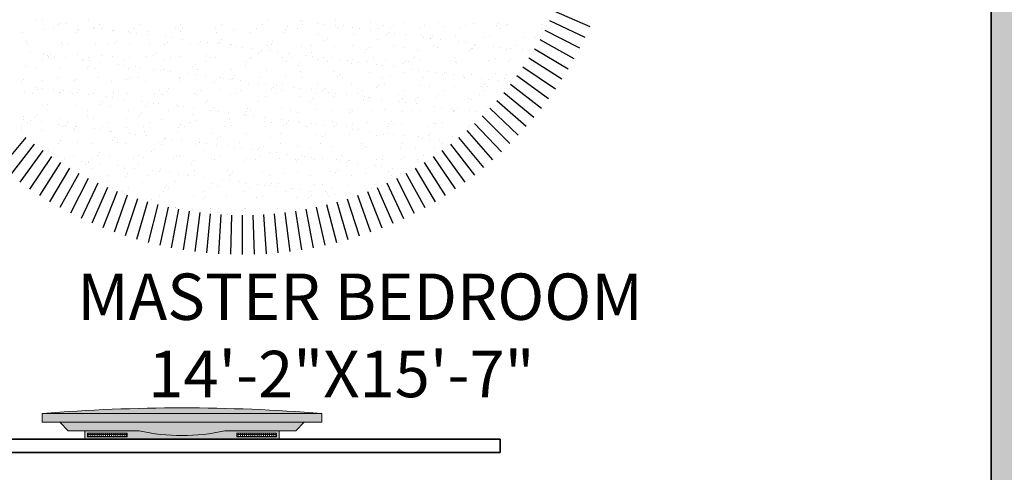
# Model space of a CAD drawing. Units: inches. Extents: x 1566 to 2546, y 1087 to 2705.
# Tile 21 of 27: x 2130 to 2278, y 1625 to 1694. Entities that reach past the tile are written whole.
import ezdxf

# ---------------------------------------------------------------- set-up
doc = ezdxf.new("R2010")
doc.units = ezdxf.units.IN
for name, color, linetype, lineweight in [('A-AREA-IDEN', 7, 'Continuous', 18), ('A-FURN', 8, 'Continuous', 18), ('A-WALL', 7, 'Continuous', 35), ('A-WALL-PATT', 8, 'Continuous', 13), ('moveis', 254, 'Continuous', 5), ('parede', 7, 'Continuous', 30)]:
    doc.layers.add(name, color=color, linetype=linetype, lineweight=lineweight)
doc.layers.add('A-HT', color=15, linetype='Continuous')
doc.styles.get("Standard").update_dxf_attribs({"font": 'arial.ttf'})

# ---------------------------------------------------------------- blocks, each defined once
blk = doc.blocks.new('*X21')
at = {"color": 0}
for p, q in [((1.8017, 2.833), (1.8017, 2.833)), ((1.8783, 2.8364), (1.8783, 2.8364)), ((1.9044, 2.8399), (1.9044, 2.8399)), ((1.945, 2.8452), (1.945, 2.8452)), ((2.0018, 2.8313), (2.0018, 2.8313)), ((1.7428, 2.8186), (1.7428, 2.8186)), ((1.7438, 2.8187), (1.7438, 2.8187)), ((1.7537, 2.8227), (1.7537, 2.8227)), ((1.7698, 2.8221), (1.7698, 2.8221)), ((1.8104, 2.8275), (1.8104, 2.8275)), ((1.8778, 2.8235), (1.8778, 2.8235)), ((1.9094, 2.823), (1.9094, 2.823)), ((2.0087, 2.8252), (2.0087, 2.8252)), ((2.011, 2.8229), (2.011, 2.8229)), ((2.0652, 2.8233), (2.0652, 2.8233)), ((2.1366, 2.8246), (2.1366, 2.8246)), ((2.2048, 2.8269), (2.2048, 2.8269)), ((2.2209, 2.8236), (2.2209, 2.8236)), ((1.5414, 2.759), (1.5414, 2.759)), ((1.5474, 2.7675), (1.5474, 2.7675)), ((1.6514, 2.7891), (1.6514, 2.7891)), ((1.6825, 2.7724), (1.6825, 2.7724)), ((1.6971, 2.7593), (1.6971, 2.7593)), ((1.8133, 2.774), (1.8133, 2.774)), ((1.8515, 2.7874), (1.8515, 2.7874)), ((1.8528, 2.7596), (1.8528, 2.7596)), ((1.8607, 2.779), (1.8607, 2.779)), ((1.9412, 2.7734), (1.9412, 2.7734)), ((2.0085, 2.7599), (2.0085, 2.7599)), ((2.0545, 2.783), (2.0545, 2.783)), ((2.0763, 2.7783), (2.0763, 2.7783)), ((2.1643, 2.7602), (2.1643, 2.7602)), ((2.2072, 2.78), (2.2072, 2.78)), ((2.2546, 2.7813), (2.2546, 2.7813)), ((2.2603, 2.7573), (2.2603, 2.7573)), ((2.2638, 2.7728), (2.2638, 2.7728)), ((2.32, 2.7605), (2.32, 2.7605)), ((2.3282, 2.7662), (2.3282, 2.7662)), ((2.3351, 2.7793), (2.3351, 2.7793)), ((2.3542, 2.7696), (2.3542, 2.7696)), ((2.3949, 2.775), (2.3949, 2.775)), ((1.4871, 2.7212), (1.4871, 2.7212)), ((1.5011, 2.7453), (1.5011, 2.7453)), ((1.5625, 2.7456), (1.5625, 2.7456)), ((1.618, 2.7229), (1.618, 2.7229)), ((1.7012, 2.7435), (1.7012, 2.7435)), ((1.7104, 2.7351), (1.7104, 2.7351)), ((1.7182, 2.7459), (1.7182, 2.7459)), ((1.7459, 2.7223), (1.7459, 2.7223)), ((1.8739, 2.7462), (1.8739, 2.7462)), ((1.881, 2.7272), (1.881, 2.7272)), ((1.9042, 2.7391), (1.9042, 2.7391)), ((1.9505, 2.7165), (1.9505, 2.7165)), ((1.9911, 2.7218), (1.9911, 2.7218)), ((2.0118, 2.7288), (2.0118, 2.7288)), ((2.0296, 2.7465), (2.0296, 2.7465)), ((2.059, 2.7308), (2.059, 2.7308)), ((2.0851, 2.7342), (2.0851, 2.7342)), ((2.1043, 2.7374), (2.1043, 2.7374)), ((2.1135, 2.729), (2.1135, 2.729)), ((2.1257, 2.7395), (2.1257, 2.7395)), ((2.1397, 2.7282), (2.1397, 2.7282)), ((2.1853, 2.7467), (2.1853, 2.7467)), ((2.1936, 2.7485), (2.1936, 2.7485)), ((2.2196, 2.7519), (2.2196, 2.7519)), ((2.2748, 2.7331), (2.2748, 2.7331)), ((2.3073, 2.733), (2.3073, 2.733)), ((2.341, 2.747), (2.341, 2.747)), ((2.4057, 2.7348), (2.4057, 2.7348)), ((2.4967, 2.7473), (2.4967, 2.7473)), ((2.5074, 2.7313), (2.5074, 2.7313)), ((2.5166, 2.7228), (2.5166, 2.7228)), ((2.5336, 2.7341), (2.5336, 2.7341)), ((1.4827, 2.697), (1.4827, 2.697)), ((1.5509, 2.6997), (1.5509, 2.6997)), ((1.5601, 2.6912), (1.5601, 2.6912)), ((1.6384, 2.6973), (1.6384, 2.6973)), ((1.6553, 2.6776), (1.6553, 2.6776)), ((1.6813, 2.681), (1.6813, 2.681)), ((1.7219, 2.6864), (1.7219, 2.6864)), ((1.7539, 2.6952), (1.7539, 2.6952)), ((1.7899, 2.6953), (1.7899, 2.6953)), ((1.7941, 2.6975), (1.7941, 2.6975)), ((1.8159, 2.6988), (1.8159, 2.6988)), ((1.8165, 2.6777), (1.8165, 2.6777)), ((1.8565, 2.7041), (1.8565, 2.7041)), ((1.9244, 2.7131), (1.9244, 2.7131)), ((1.9498, 2.6978), (1.9498, 2.6978)), ((1.954, 2.6935), (1.954, 2.6935)), ((1.9632, 2.6851), (1.9632, 2.6851)), ((2.0794, 2.682), (2.0794, 2.682)), ((2.1055, 2.6981), (2.1055, 2.6981)), ((2.157, 2.6891), (2.157, 2.6891)), ((2.2103, 2.6836), (2.2103, 2.6836)), ((2.2612, 2.6984), (2.2612, 2.6984)), ((2.3382, 2.683), (2.3382, 2.683)), ((2.3571, 2.6874), (2.3571, 2.6874)), ((2.3663, 2.6789), (2.3663, 2.6789)), ((2.4169, 2.6987), (2.4169, 2.6987)), ((2.4733, 2.6879), (2.4733, 2.6879)), ((2.5601, 2.683), (2.5601, 2.683)), ((2.5727, 2.6989), (2.5727, 2.6989)), ((2.6042, 2.6895), (2.6042, 2.6895)), ((2.6435, 2.6783), (2.6435, 2.6783)), ((1.3861, 2.6422), (1.3861, 2.6422)), ((1.4006, 2.6558), (1.4006, 2.6558)), ((1.4098, 2.6473), (1.4098, 2.6473)), ((1.4121, 2.6456), (1.4121, 2.6456)), ((1.4227, 2.6718), (1.4227, 2.6718)), ((1.4528, 2.651), (1.4528, 2.651)), ((1.5207, 2.6599), (1.5207, 2.6599)), ((1.5467, 2.6633), (1.5467, 2.6633)), ((1.5506, 2.6712), (1.5506, 2.6712)), ((1.5873, 2.6687), (1.5873, 2.6687)), ((1.6036, 2.6513), (1.6036, 2.6513)), ((1.6856, 2.676), (1.6856, 2.676)), ((1.8037, 2.6496), (1.8037, 2.6496)), ((1.8129, 2.6412), (1.8129, 2.6412)), ((1.9444, 2.6771), (1.9444, 2.6771)), ((2.0067, 2.6452), (2.0067, 2.6452)), ((2.2068, 2.6435), (2.2068, 2.6435)), ((2.3743, 2.6428), (2.3743, 2.6428)), ((2.4003, 2.6462), (2.4003, 2.6462)), ((2.441, 2.6516), (2.441, 2.6516)), ((2.5089, 2.6605), (2.5089, 2.6605)), ((2.5349, 2.664), (2.5349, 2.664)), ((2.5756, 2.6693), (2.5756, 2.6693)), ((2.6718, 2.6427), (2.6718, 2.6427)), ((1.2503, 2.6119), (1.2503, 2.6119)), ((1.2595, 2.6034), (1.2595, 2.6034)), ((1.2775, 2.6279), (1.2775, 2.6279)), ((1.2915, 2.6198), (1.2915, 2.6198)), ((1.3182, 2.6332), (1.3182, 2.6332)), ((1.3552, 2.62), (1.3552, 2.62)), ((1.4261, 2.6336), (1.4261, 2.6336)), ((1.4472, 2.6201), (1.4472, 2.6201)), ((1.4533, 2.6075), (1.4533, 2.6075)), ((1.4903, 2.6249), (1.4903, 2.6249)), ((1.5818, 2.6338), (1.5818, 2.6338)), ((1.6029, 2.6204), (1.6029, 2.6204)), ((1.6212, 2.6266), (1.6212, 2.6266)), ((1.6534, 2.6057), (1.6534, 2.6057)), ((1.7375, 2.6341), (1.7375, 2.6341)), ((1.7491, 2.626), (1.7491, 2.626)), ((1.7586, 2.6207), (1.7586, 2.6207)), ((1.8841, 2.6308), (1.8841, 2.6308)), ((1.8932, 2.6344), (1.8932, 2.6344)), ((1.9143, 2.621), (1.9143, 2.621)), ((2.015, 2.6325), (2.015, 2.6325)), ((2.0489, 2.6347), (2.0489, 2.6347)), ((2.07, 2.6213), (2.07, 2.6213)), ((2.1051, 2.6074), (2.1051, 2.6074)), ((2.1312, 2.6108), (2.1312, 2.6108)), ((2.1429, 2.6319), (2.1429, 2.6319)), ((2.1718, 2.6162), (2.1718, 2.6162)), ((2.2046, 2.635), (2.2046, 2.635)), ((2.216, 2.635), (2.216, 2.635)), ((2.2257, 2.6215), (2.2257, 2.6215)), ((2.2397, 2.6251), (2.2397, 2.6251)), ((2.2657, 2.6285), (2.2657, 2.6285)), ((2.2779, 2.6367), (2.2779, 2.6367)), ((2.3064, 2.6339), (2.3064, 2.6339)), ((2.3603, 2.6352), (2.3603, 2.6352)), ((2.3814, 2.6218), (2.3814, 2.6218)), ((2.4088, 2.6384), (2.4088, 2.6384)), ((2.4098, 2.6391), (2.4098, 2.6391)), ((2.516, 2.6355), (2.516, 2.6355)), ((2.5367, 2.6378), (2.5367, 2.6378)), ((2.5371, 2.6221), (2.5371, 2.6221)), ((2.6099, 2.6374), (2.6099, 2.6374)), ((2.6191, 2.6289), (2.6191, 2.6289)), ((2.6718, 2.6358), (2.6718, 2.6358)), ((2.6928, 2.6224), (2.6928, 2.6224)), ((1.2117, 2.5712), (1.2117, 2.5712)), ((1.2949, 2.5738), (1.2949, 2.5738)), ((1.3674, 2.5715), (1.3674, 2.5715)), ((1.4258, 2.5754), (1.4258, 2.5754)), ((1.5231, 2.5718), (1.5231, 2.5718)), ((1.5537, 2.5748), (1.5537, 2.5748)), ((1.6626, 2.5973), (1.6626, 2.5973)), ((1.6788, 2.572), (1.6788, 2.572)), ((1.6888, 2.5797), (1.6888, 2.5797)), ((1.8196, 2.5814), (1.8196, 2.5814)), ((1.8345, 2.5723), (1.8345, 2.5723)), ((1.836, 2.5719), (1.836, 2.5719)), ((1.8564, 2.6013), (1.8564, 2.6013)), ((1.862, 2.5754), (1.862, 2.5754)), ((1.9026, 2.5807), (1.9026, 2.5807)), ((1.9475, 2.5807), (1.9475, 2.5807)), ((1.9705, 2.5897), (1.9705, 2.5897)), ((1.9902, 2.5726), (1.9902, 2.5726)), ((1.9966, 2.5931), (1.9966, 2.5931)), ((2.0372, 2.5984), (2.0372, 2.5984)), ((2.0565, 2.5996), (2.0565, 2.5996)), ((2.0657, 2.5912), (2.0657, 2.5912)), ((2.0826, 2.5856), (2.0826, 2.5856)), ((2.1459, 2.5729), (2.1459, 2.5729)), ((2.2135, 2.5873), (2.2135, 2.5873)), ((2.2595, 2.5952), (2.2595, 2.5952)), ((2.3016, 2.5732), (2.3016, 2.5732)), ((2.3414, 2.5867), (2.3414, 2.5867)), ((2.4573, 2.5735), (2.4573, 2.5735)), ((2.4595, 2.5935), (2.4595, 2.5935)), ((2.4688, 2.585), (2.4688, 2.585)), ((2.4764, 2.5915), (2.4764, 2.5915)), ((2.6073, 2.5932), (2.6073, 2.5932)), ((2.613, 2.5737), (2.613, 2.5737)), ((2.6626, 2.589), (2.6626, 2.589)), ((2.7352, 2.5926), (2.7352, 2.5926)), ((2.7687, 2.574), (2.7687, 2.574)), ((1.303, 2.5636), (1.303, 2.5636)), ((1.4934, 2.5286), (1.4934, 2.5286)), ((1.4989, 2.5276), (1.4989, 2.5276)), ((1.5031, 2.5619), (1.5031, 2.5619)), ((1.5123, 2.5534), (1.5123, 2.5534)), ((1.5668, 2.5365), (1.5668, 2.5365)), ((1.5928, 2.5399), (1.5928, 2.5399)), ((1.6243, 2.5302), (1.6243, 2.5302)), ((1.6334, 2.5453), (1.6334, 2.5453)), ((1.7014, 2.5542), (1.7014, 2.5542)), ((1.7061, 2.5574), (1.7061, 2.5574)), ((1.7274, 2.5577), (1.7274, 2.5577)), ((1.7522, 2.5296), (1.7522, 2.5296)), ((1.768, 2.563), (1.768, 2.563)), ((1.8873, 2.5345), (1.8873, 2.5345)), ((1.9061, 2.5557), (1.9061, 2.5557)), ((1.9154, 2.5473), (1.9154, 2.5473)), ((2.0181, 2.5361), (2.0181, 2.5361)), ((2.1092, 2.5513), (2.1092, 2.5513)), ((2.146, 2.5355), (2.146, 2.5355)), ((2.2811, 2.5404), (2.2811, 2.5404)), ((2.3092, 2.5496), (2.3092, 2.5496)), ((2.3185, 2.5411), (2.3185, 2.5411)), ((2.412, 2.5421), (2.412, 2.5421)), ((2.4871, 2.5282), (2.4871, 2.5282)), ((2.5123, 2.5452), (2.5123, 2.5452)), ((2.5399, 2.5415), (2.5399, 2.5415)), ((2.555, 2.5371), (2.555, 2.5371)), ((2.581, 2.5406), (2.581, 2.5406)), ((2.6217, 2.5459), (2.6217, 2.5459)), ((2.6749, 2.5463), (2.6749, 2.5463)), ((2.6896, 2.5549), (2.6896, 2.5549)), ((2.7123, 2.5434), (2.7123, 2.5434)), ((2.7156, 2.5583), (2.7156, 2.5583)), ((2.7216, 2.535), (2.7216, 2.535)), ((2.7563, 2.5636), (2.7563, 2.5636)), ((2.8058, 2.548), (2.8058, 2.548)), ((1.1527, 2.5197), (1.1527, 2.5197)), ((1.1551, 2.5078), (1.1551, 2.5078)), ((1.1761, 2.4943), (1.1761, 2.4943)), ((1.2297, 2.4921), (1.2297, 2.4921)), ((1.2305, 2.5243), (1.2305, 2.5243)), ((1.2976, 2.5011), (1.2976, 2.5011)), ((1.3108, 2.5081), (1.3108, 2.5081)), ((1.3236, 2.5045), (1.3236, 2.5045)), ((1.3319, 2.4946), (1.3319, 2.4946)), ((1.3527, 2.518), (1.3527, 2.518)), ((1.3584, 2.5237), (1.3584, 2.5237)), ((1.362, 2.5095), (1.362, 2.5095)), ((1.3643, 2.5098), (1.3643, 2.5098)), ((1.4322, 2.5188), (1.4322, 2.5188)), ((1.4582, 2.5222), (1.4582, 2.5222)), ((1.4665, 2.5083), (1.4665, 2.5083)), ((1.4876, 2.4949), (1.4876, 2.4949)), ((1.5558, 2.5136), (1.5558, 2.5136)), ((1.6222, 2.5086), (1.6222, 2.5086)), ((1.6433, 2.4952), (1.6433, 2.4952)), ((1.7558, 2.5118), (1.7558, 2.5118)), ((1.7651, 2.5034), (1.7651, 2.5034)), ((1.7779, 2.5089), (1.7779, 2.5089)), ((1.799, 2.4955), (1.799, 2.4955)), ((1.9336, 2.5092), (1.9336, 2.5092)), ((1.9547, 2.4958), (1.9547, 2.4958)), ((1.9589, 2.5074), (1.9589, 2.5074)), ((2.0857, 2.4893), (2.0857, 2.4893)), ((2.0893, 2.5095), (2.0893, 2.5095)), ((2.1104, 2.496), (2.1104, 2.496)), ((2.1589, 2.5057), (2.1589, 2.5057)), ((2.1682, 2.4973), (2.1682, 2.4973)), ((2.2166, 2.4909), (2.2166, 2.4909)), ((2.2179, 2.4928), (2.2179, 2.4928)), ((2.245, 2.5098), (2.245, 2.5098)), ((2.2661, 2.4963), (2.2661, 2.4963)), ((2.2858, 2.5017), (2.2858, 2.5017)), ((2.3118, 2.5051), (2.3118, 2.5051)), ((2.3445, 2.4903), (2.3445, 2.4903)), ((2.3525, 2.5105), (2.3525, 2.5105)), ((2.362, 2.5013), (2.362, 2.5013)), ((2.4007, 2.51), (2.4007, 2.51)), ((2.4204, 2.5194), (2.4204, 2.5194)), ((2.4218, 2.4966), (2.4218, 2.4966)), ((2.4464, 2.5229), (2.4464, 2.5229)), ((2.4796, 2.4952), (2.4796, 2.4952)), ((2.5564, 2.5103), (2.5564, 2.5103)), ((2.562, 2.4996), (2.562, 2.4996)), ((2.5712, 2.4911), (2.5712, 2.4911)), ((2.5775, 2.4969), (2.5775, 2.4969)), ((2.6104, 2.4969), (2.6104, 2.4969)), ((2.7121, 2.5106), (2.7121, 2.5106)), ((2.7332, 2.4972), (2.7332, 2.4972)), ((2.7384, 2.4962), (2.7384, 2.4962)), ((2.7651, 2.4951), (2.7651, 2.4951)), ((2.8678, 2.5109), (2.8678, 2.5109)), ((2.8734, 2.5011), (2.8734, 2.5011)), ((2.8889, 2.4975), (2.8889, 2.4975)), ((1.163, 2.4833), (1.163, 2.4833)), ((1.163, 2.4726), (1.163, 2.4726)), ((1.189, 2.4868), (1.189, 2.4868)), ((1.2024, 2.4741), (1.2024, 2.4741)), ((1.2117, 2.4657), (1.2117, 2.4657)), ((1.2981, 2.4774), (1.2981, 2.4774)), ((1.4055, 2.4697), (1.4055, 2.4697)), ((1.429, 2.4791), (1.429, 2.4791)), ((1.5569, 2.4785), (1.5569, 2.4785)), ((1.6055, 2.468), (1.6055, 2.468)), ((1.6148, 2.4595), (1.6148, 2.4595)), ((1.6919, 2.4833), (1.6919, 2.4833)), ((1.8086, 2.4635), (1.8086, 2.4635)), ((1.8228, 2.485), (1.8228, 2.485)), ((1.9081, 2.452), (1.9081, 2.452)), ((1.9487, 2.4573), (1.9487, 2.4573)), ((1.9507, 2.4844), (1.9507, 2.4844)), ((2.0086, 2.4618), (2.0086, 2.4618)), ((2.0166, 2.4663), (2.0166, 2.4663)), ((2.0178, 2.4534), (2.0178, 2.4534)), ((2.0427, 2.4697), (2.0427, 2.4697)), ((2.0833, 2.4751), (2.0833, 2.4751)), ((2.1512, 2.484), (2.1512, 2.484)), ((2.1773, 2.4874), (2.1773, 2.4874)), ((2.2117, 2.4574), (2.2117, 2.4574)), ((2.4117, 2.4557), (2.4117, 2.4557)), ((2.8089, 2.4516), (2.8089, 2.4516)), ((2.8963, 2.4526), (2.8963, 2.4526)), ((1.2336, 2.428), (1.2336, 2.428)), ((1.2521, 2.446), (1.2521, 2.446)), ((1.2552, 2.4258), (1.2552, 2.4258)), ((1.3615, 2.4273), (1.3615, 2.4273)), ((1.4078, 2.4463), (1.4078, 2.4463)), ((1.4552, 2.4241), (1.4552, 2.4241)), ((1.4644, 2.4156), (1.4644, 2.4156)), ((1.4966, 2.4322), (1.4966, 2.4322)), ((1.5635, 2.4466), (1.5635, 2.4466)), ((1.6275, 2.4339), (1.6275, 2.4339)), ((1.6389, 2.4165), (1.6389, 2.4165)), ((1.6582, 2.4197), (1.6582, 2.4197)), ((1.6795, 2.4219), (1.6795, 2.4219)), ((1.7192, 2.4468), (1.7192, 2.4468)), ((1.7475, 2.4308), (1.7475, 2.4308)), ((1.7554, 2.4333), (1.7554, 2.4333)), ((1.7735, 2.4343), (1.7735, 2.4343)), ((1.8141, 2.4396), (1.8141, 2.4396)), ((1.8583, 2.4179), (1.8583, 2.4179)), ((1.8749, 2.4471), (1.8749, 2.4471)), ((1.8821, 2.4486), (1.8821, 2.4486)), ((1.8904, 2.4381), (1.8904, 2.4381)), ((2.0213, 2.4398), (2.0213, 2.4398)), ((2.0306, 2.4474), (2.0306, 2.4474)), ((2.1492, 2.4392), (2.1492, 2.4392)), ((2.1863, 2.4477), (2.1863, 2.4477)), ((2.2842, 2.4441), (2.2842, 2.4441)), ((2.342, 2.448), (2.342, 2.448)), ((2.4151, 2.4457), (2.4151, 2.4457)), ((2.4209, 2.4472), (2.4209, 2.4472)), ((2.4977, 2.4483), (2.4977, 2.4483)), ((2.543, 2.4451), (2.543, 2.4451)), ((2.6011, 2.4138), (2.6011, 2.4138)), ((2.6147, 2.4513), (2.6147, 2.4513)), ((2.6271, 2.4172), (2.6271, 2.4172)), ((2.6534, 2.4485), (2.6534, 2.4485)), ((2.6678, 2.4225), (2.6678, 2.4225)), ((2.6781, 2.45), (2.6781, 2.45)), ((2.7357, 2.4315), (2.7357, 2.4315)), ((2.7617, 2.4349), (2.7617, 2.4349)), ((2.8024, 2.4403), (2.8024, 2.4403)), ((2.8091, 2.4488), (2.8091, 2.4488)), ((2.8148, 2.4495), (2.8148, 2.4495)), ((2.824, 2.4411), (2.824, 2.4411)), ((2.8703, 2.4492), (2.8703, 2.4492)), ((2.9368, 2.451), (2.9368, 2.451)), ((1.1662, 2.3762), (1.1662, 2.3762)), ((1.1954, 2.3826), (1.1954, 2.3826)), ((1.3012, 2.3811), (1.3012, 2.3811)), ((1.3049, 2.3802), (1.3049, 2.3802)), ((1.3437, 2.3777), (1.3437, 2.3777)), ((1.3512, 2.3829), (1.3512, 2.3829)), ((1.3697, 2.3811), (1.3697, 2.3811)), ((1.4104, 2.3865), (1.4104, 2.3865)), ((1.4321, 2.3828), (1.4321, 2.3828)), ((1.4783, 2.3954), (1.4783, 2.3954)), ((1.5043, 2.3988), (1.5043, 2.3988)), ((1.5069, 2.3831), (1.5069, 2.3831)), ((1.545, 2.4042), (1.545, 2.4042)), ((1.56, 2.3821), (1.56, 2.3821)), ((1.6129, 2.4131), (1.6129, 2.4131)), ((1.6626, 2.3834), (1.6626, 2.3834)), ((1.6951, 2.387), (1.6951, 2.387)), ((1.8183, 2.3837), (1.8183, 2.3837)), ((1.8259, 2.3887), (1.8259, 2.3887)), ((1.8675, 2.4095), (1.8675, 2.4095)), ((1.9538, 2.3881), (1.9538, 2.3881)), ((1.974, 2.384), (1.974, 2.384)), ((2.0613, 2.4135), (2.0613, 2.4135)), ((2.0889, 2.3929), (2.0889, 2.3929)), ((2.1297, 2.3843), (2.1297, 2.3843)), ((2.2198, 2.3946), (2.2198, 2.3946)), ((2.2614, 2.4118), (2.2614, 2.4118)), ((2.2706, 2.4033), (2.2706, 2.4033)), ((2.2854, 2.3846), (2.2854, 2.3846)), ((2.3319, 2.3783), (2.3319, 2.3783)), ((2.3477, 2.394), (2.3477, 2.394)), ((2.3579, 2.3817), (2.3579, 2.3817)), ((2.3986, 2.3871), (2.3986, 2.3871)), ((2.4411, 2.3848), (2.4411, 2.3848)), ((2.4644, 2.4074), (2.4644, 2.4074)), ((2.4665, 2.396), (2.4665, 2.396)), ((2.4827, 2.3988), (2.4827, 2.3988)), ((2.4925, 2.3995), (2.4925, 2.3995)), ((2.5332, 2.4048), (2.5332, 2.4048)), ((2.5968, 2.3851), (2.5968, 2.3851)), ((2.6136, 2.4005), (2.6136, 2.4005)), ((2.6645, 2.4057), (2.6645, 2.4057)), ((2.6737, 2.3972), (2.6737, 2.3972)), ((2.7415, 2.3999), (2.7415, 2.3999)), ((2.7525, 2.3854), (2.7525, 2.3854)), ((2.8675, 2.4012), (2.8675, 2.4012)), ((2.8765, 2.4048), (2.8765, 2.4048)), ((2.9082, 2.3857), (2.9082, 2.3857)), ((1.2091, 2.36), (1.2091, 2.36)), ((1.2165, 2.3691), (1.2165, 2.3691)), ((1.2351, 2.3634), (1.2351, 2.3634)), ((1.2758, 2.3687), (1.2758, 2.3687)), ((1.3141, 2.3717), (1.3141, 2.3717)), ((1.3722, 2.3694), (1.3722, 2.3694)), ((1.5079, 2.3758), (1.5079, 2.3758)), ((1.5279, 2.3697), (1.5279, 2.3697)), ((1.6837, 2.37), (1.6837, 2.37)), ((1.708, 2.374), (1.708, 2.374)), ((1.7172, 2.3656), (1.7172, 2.3656)), ((1.8394, 2.3703), (1.8394, 2.3703)), ((1.8936, 2.3418), (1.8936, 2.3418)), ((1.911, 2.3696), (1.911, 2.3696)), ((1.9951, 2.3706), (1.9951, 2.3706)), ((2.0244, 2.3435), (2.0244, 2.3435)), ((2.0627, 2.3429), (2.0627, 2.3429)), ((2.0888, 2.3463), (2.0888, 2.3463)), ((2.1111, 2.3679), (2.1111, 2.3679)), ((2.1203, 2.3595), (2.1203, 2.3595)), ((2.1294, 2.3517), (2.1294, 2.3517)), ((2.1508, 2.3708), (2.1508, 2.3708)), ((2.1523, 2.3429), (2.1523, 2.3429)), ((2.1973, 2.3606), (2.1973, 2.3606)), ((2.2234, 2.364), (2.2234, 2.364)), ((2.264, 2.3694), (2.264, 2.3694)), ((2.2874, 2.3477), (2.2874, 2.3477)), ((2.3065, 2.3711), (2.3065, 2.3711)), ((2.3141, 2.3635), (2.3141, 2.3635)), ((2.4183, 2.3494), (2.4183, 2.3494)), ((2.4622, 2.3714), (2.4622, 2.3714)), ((2.5142, 2.3618), (2.5142, 2.3618)), ((2.5234, 2.3533), (2.5234, 2.3533)), ((2.5462, 2.3488), (2.5462, 2.3488)), ((2.6179, 2.3717), (2.6179, 2.3717)), ((2.6812, 2.3536), (2.6812, 2.3536)), ((2.7172, 2.3573), (2.7172, 2.3573)), ((2.7736, 2.372), (2.7736, 2.372)), ((2.8121, 2.3553), (2.8121, 2.3553)), ((2.9173, 2.3556), (2.9173, 2.3556)), ((2.9265, 2.3472), (2.9265, 2.3472)), ((2.9293, 2.3723), (2.9293, 2.3723)), ((2.94, 2.3547), (2.94, 2.3547)), ((1.1546, 2.3363), (1.1546, 2.3363)), ((1.1638, 2.3279), (1.1638, 2.3279)), ((1.2368, 2.3316), (1.2368, 2.3316)), ((1.2924, 2.3208), (1.2924, 2.3208)), ((1.3576, 2.3319), (1.3576, 2.3319)), ((1.3647, 2.331), (1.3647, 2.331)), ((1.4481, 2.3211), (1.4481, 2.3211)), ((1.4997, 2.3359), (1.4997, 2.3359)), ((1.5577, 2.3302), (1.5577, 2.3302)), ((1.5669, 2.3217), (1.5669, 2.3217)), ((1.6038, 2.3214), (1.6038, 2.3214)), ((1.6306, 2.3375), (1.6306, 2.3375)), ((1.7585, 2.3369), (1.7585, 2.3369)), ((1.7596, 2.3216), (1.7596, 2.3216)), ((1.7607, 2.3257), (1.7607, 2.3257)), ((1.7936, 2.3074), (1.7936, 2.3074)), ((1.8196, 2.3109), (1.8196, 2.3109)), ((1.8602, 2.3162), (1.8602, 2.3162)), ((1.9153, 2.3219), (1.9153, 2.3219)), ((1.9282, 2.3252), (1.9282, 2.3252)), ((1.9542, 2.3286), (1.9542, 2.3286)), ((1.9608, 2.324), (1.9608, 2.324)), ((1.97, 2.3156), (1.97, 2.3156)), ((1.9948, 2.3339), (1.9948, 2.3339)), ((2.071, 2.3222), (2.071, 2.3222)), ((2.1638, 2.3196), (2.1638, 2.3196)), ((2.2267, 2.3225), (2.2267, 2.3225)), ((2.3639, 2.3179), (2.3639, 2.3179)), ((2.3731, 2.3094), (2.3731, 2.3094)), ((2.3824, 2.3228), (2.3824, 2.3228)), ((2.4859, 2.3025), (2.4859, 2.3025)), ((2.5381, 2.323), (2.5381, 2.323)), ((2.5669, 2.3135), (2.5669, 2.3135)), ((2.6167, 2.3042), (2.6167, 2.3042)), ((2.6938, 2.3233), (2.6938, 2.3233)), ((2.7447, 2.3036), (2.7447, 2.3036)), ((2.767, 2.3117), (2.767, 2.3117)), ((2.7762, 2.3033), (2.7762, 2.3033)), ((2.7818, 2.3081), (2.7818, 2.3081)), ((2.8078, 2.3115), (2.8078, 2.3115)), ((2.8485, 2.3169), (2.8485, 2.3169)), ((2.8495, 2.3236), (2.8495, 2.3236)), ((2.8797, 2.3084), (2.8797, 2.3084)), ((2.9164, 2.3258), (2.9164, 2.3258)), ((2.9424, 2.3292), (2.9424, 2.3292)), ((2.97, 2.3073), (2.97, 2.3073)), ((2.983, 2.3346), (2.983, 2.3346)), ((3.0052, 2.3239), (3.0052, 2.3239)), ((3.0106, 2.3101), (3.0106, 2.3101)), ((1.1693, 2.2799), (1.1693, 2.2799)), ((1.2073, 2.288), (1.2073, 2.288)), ((1.3044, 2.2847), (1.3044, 2.2847)), ((1.4074, 2.2863), (1.4074, 2.2863)), ((1.4166, 2.2778), (1.4166, 2.2778)), ((1.4353, 2.2864), (1.4353, 2.2864)), ((1.4565, 2.2631), (1.4565, 2.2631)), ((1.5244, 2.272), (1.5244, 2.272)), ((1.5504, 2.2754), (1.5504, 2.2754)), ((1.5632, 2.2858), (1.5632, 2.2858)), ((1.5911, 2.2808), (1.5911, 2.2808)), ((1.6104, 2.2819), (1.6104, 2.2819)), ((1.659, 2.2897), (1.659, 2.2897)), ((1.685, 2.2932), (1.685, 2.2932)), ((1.6982, 2.2907), (1.6982, 2.2907)), ((1.7256, 2.2985), (1.7256, 2.2985)), ((1.8105, 2.2801), (1.8105, 2.2801)), ((1.8197, 2.2717), (1.8197, 2.2717)), ((1.8291, 2.2923), (1.8291, 2.2923)), ((1.957, 2.2917), (1.957, 2.2917)), ((2.0135, 2.2757), (2.0135, 2.2757)), ((2.092, 2.2966), (2.092, 2.2966)), ((2.2136, 2.274), (2.2136, 2.274)), ((2.2228, 2.2656), (2.2228, 2.2656)), ((2.2229, 2.2983), (2.2229, 2.2983)), ((2.3508, 2.2976), (2.3508, 2.2976)), ((2.4166, 2.2696), (2.4166, 2.2696)), ((2.4447, 2.2637), (2.4447, 2.2637)), ((2.5126, 2.2727), (2.5126, 2.2727)), ((2.5386, 2.2761), (2.5386, 2.2761)), ((2.5793, 2.2814), (2.5793, 2.2814)), ((2.6167, 2.2679), (2.6167, 2.2679)), ((2.6472, 2.2904), (2.6472, 2.2904)), ((2.6732, 2.2938), (2.6732, 2.2938)), ((2.7139, 2.2992), (2.7139, 2.2992)), ((2.8197, 2.2634), (2.8197, 2.2634)), ((3.0782, 2.2632), (3.0782, 2.2632)), ((1.1873, 2.2276), (1.1873, 2.2276)), ((1.2358, 2.2574), (1.2358, 2.2574)), ((1.2399, 2.2353), (1.2399, 2.2353)), ((1.2552, 2.2366), (1.2552, 2.2366)), ((1.2569, 2.2439), (1.2569, 2.2439)), ((1.2571, 2.2424), (1.2571, 2.2424)), ((1.2663, 2.234), (1.2663, 2.234)), ((1.2812, 2.24), (1.2812, 2.24)), ((1.3219, 2.2453), (1.3219, 2.2453)), ((1.3678, 2.2347), (1.3678, 2.2347)), ((1.3898, 2.2543), (1.3898, 2.2543)), ((1.3915, 2.2577), (1.3915, 2.2577)), ((1.4126, 2.2442), (1.4126, 2.2442)), ((1.4158, 2.2577), (1.4158, 2.2577)), ((1.4601, 2.238), (1.4601, 2.238)), ((1.5029, 2.2395), (1.5029, 2.2395)), ((1.5472, 2.2579), (1.5472, 2.2579)), ((1.5683, 2.2445), (1.5683, 2.2445)), ((1.6338, 2.2412), (1.6338, 2.2412)), ((1.6602, 2.2363), (1.6602, 2.2363)), ((1.6694, 2.2278), (1.6694, 2.2278)), ((1.7029, 2.2582), (1.7029, 2.2582)), ((1.724, 2.2448), (1.724, 2.2448)), ((1.7617, 2.2406), (1.7617, 2.2406)), ((1.8587, 2.2585), (1.8587, 2.2585)), ((1.8632, 2.2318), (1.8632, 2.2318)), ((1.8797, 2.2451), (1.8797, 2.2451)), ((1.8967, 2.2455), (1.8967, 2.2455)), ((2.0144, 2.2588), (2.0144, 2.2588)), ((2.0276, 2.2471), (2.0276, 2.2471)), ((2.0354, 2.2454), (2.0354, 2.2454)), ((2.0633, 2.2301), (2.0633, 2.2301)), ((2.1555, 2.2465), (2.1555, 2.2465)), ((2.1701, 2.2591), (2.1701, 2.2591)), ((2.1755, 2.2283), (2.1755, 2.2283)), ((2.1912, 2.2456), (2.1912, 2.2456)), ((2.2434, 2.2372), (2.2434, 2.2372)), ((2.2663, 2.2257), (2.2663, 2.2257)), ((2.2695, 2.2406), (2.2695, 2.2406)), ((2.2905, 2.2514), (2.2905, 2.2514)), ((2.3101, 2.246), (2.3101, 2.246)), ((2.3258, 2.2594), (2.3258, 2.2594)), ((2.3469, 2.2459), (2.3469, 2.2459)), ((2.378, 2.2549), (2.378, 2.2549)), ((2.404, 2.2584), (2.404, 2.2584)), ((2.4214, 2.253), (2.4214, 2.253)), ((2.4815, 2.2596), (2.4815, 2.2596)), ((2.5026, 2.2462), (2.5026, 2.2462)), ((2.5493, 2.2524), (2.5493, 2.2524)), ((2.6259, 2.2594), (2.6259, 2.2594)), ((2.6372, 2.2599), (2.6372, 2.2599)), ((2.6583, 2.2465), (2.6583, 2.2465)), ((2.6844, 2.2573), (2.6844, 2.2573)), ((2.7929, 2.2602), (2.7929, 2.2602)), ((2.814, 2.2468), (2.814, 2.2468)), ((2.8152, 2.259), (2.8152, 2.259)), ((2.9431, 2.2584), (2.9431, 2.2584)), ((2.9486, 2.2605), (2.9486, 2.2605)), ((2.9697, 2.2471), (2.9697, 2.2471)), ((3.0198, 2.2617), (3.0198, 2.2617)), ((3.029, 2.2533), (3.029, 2.2533)), ((1.1771, 2.1953), (1.1771, 2.1953)), ((1.3075, 2.1884), (1.3075, 2.1884)), ((1.3098, 2.1941), (1.3098, 2.1941)), ((1.3328, 2.1956), (1.3328, 2.1956)), ((1.4384, 2.1901), (1.4384, 2.1901)), ((1.4885, 2.1959), (1.4885, 2.1959)), ((1.5099, 2.1924), (1.5099, 2.1924)), ((1.5663, 2.1895), (1.5663, 2.1895)), ((1.6442, 2.1961), (1.6442, 2.1961)), ((1.7014, 2.1943), (1.7014, 2.1943)), ((1.7129, 2.188), (1.7129, 2.188)), ((1.7999, 2.1964), (1.7999, 2.1964)), ((1.8322, 2.196), (1.8322, 2.196)), ((1.8657, 2.1875), (1.8657, 2.1875)), ((1.9063, 2.1928), (1.9063, 2.1928)), ((1.9556, 2.1967), (1.9556, 2.1967)), ((1.9601, 2.1954), (1.9601, 2.1954)), ((1.9743, 2.2018), (1.9743, 2.2018)), ((2.0003, 2.2052), (2.0003, 2.2052)), ((2.0409, 2.2106), (2.0409, 2.2106)), ((2.0725, 2.2217), (2.0725, 2.2217)), ((2.0952, 2.2002), (2.0952, 2.2002)), ((2.1088, 2.2195), (2.1088, 2.2195)), ((2.1114, 2.197), (2.1114, 2.197)), ((2.1349, 2.2229), (2.1349, 2.2229)), ((2.2261, 2.2019), (2.2261, 2.2019)), ((2.2671, 2.1973), (2.2671, 2.1973)), ((2.354, 2.2013), (2.354, 2.2013)), ((2.4228, 2.1976), (2.4228, 2.1976)), ((2.4664, 2.224), (2.4664, 2.224)), ((2.4756, 2.2155), (2.4756, 2.2155)), ((2.489, 2.2062), (2.489, 2.2062)), ((2.5785, 2.1978), (2.5785, 2.1978)), ((2.6199, 2.2078), (2.6199, 2.2078)), ((2.6694, 2.2196), (2.6694, 2.2196)), ((2.7342, 2.1981), (2.7342, 2.1981)), ((2.7478, 2.2072), (2.7478, 2.2072)), ((2.8539, 2.1881), (2.8539, 2.1881)), ((2.8695, 2.2178), (2.8695, 2.2178)), ((2.8787, 2.2094), (2.8787, 2.2094)), ((2.8828, 2.2121), (2.8828, 2.2121)), ((2.8899, 2.1984), (2.8899, 2.1984)), ((2.8946, 2.1935), (2.8946, 2.1935)), ((2.9625, 2.2024), (2.9625, 2.2024)), ((2.9885, 2.2058), (2.9885, 2.2058)), ((3.0137, 2.2138), (3.0137, 2.2138)), ((3.0291, 2.2112), (3.0291, 2.2112)), ((3.0456, 2.1987), (3.0456, 2.1987)), ((3.0725, 2.2134), (3.0725, 2.2134)), ((3.0971, 2.2201), (3.0971, 2.2201)), ((1.1595, 2.1502), (1.1595, 2.1502)), ((1.1725, 2.1835), (1.1725, 2.1835)), ((1.5191, 2.1839), (1.5191, 2.1839)), ((1.5965, 2.152), (1.5965, 2.152)), ((1.6372, 2.1574), (1.6372, 2.1574)), ((1.7051, 2.1663), (1.7051, 2.1663)), ((1.7311, 2.1698), (1.7311, 2.1698)), ((1.7717, 2.1751), (1.7717, 2.1751)), ((1.8397, 2.1841), (1.8397, 2.1841)), ((1.913, 2.1862), (1.913, 2.1862)), ((1.9222, 2.1778), (1.9222, 2.1778)), ((2.0307, 2.1508), (2.0307, 2.1508)), ((2.116, 2.1818), (2.116, 2.1818)), ((2.1586, 2.1502), (2.1586, 2.1502)), ((2.2937, 2.155), (2.2937, 2.155)), ((2.3161, 2.1801), (2.3161, 2.1801)), ((2.3253, 2.1717), (2.3253, 2.1717)), ((2.4246, 2.1567), (2.4246, 2.1567)), ((2.5191, 2.1757), (2.5191, 2.1757)), ((2.5525, 2.1561), (2.5525, 2.1561)), ((2.5847, 2.1527), (2.5847, 2.1527)), ((2.6254, 2.158), (2.6254, 2.158)), ((2.6875, 2.161), (2.6875, 2.161)), ((2.6933, 2.167), (2.6933, 2.167)), ((2.7192, 2.174), (2.7192, 2.174)), ((2.7193, 2.1704), (2.7193, 2.1704)), ((2.7284, 2.1655), (2.7284, 2.1655)), ((2.76, 2.1758), (2.76, 2.1758)), ((2.8184, 2.1626), (2.8184, 2.1626)), ((2.8279, 2.1847), (2.8279, 2.1847)), ((2.9222, 2.1695), (2.9222, 2.1695)), ((2.9463, 2.162), (2.9463, 2.162)), ((3.0813, 2.1669), (3.0813, 2.1669)), ((3.1223, 2.1678), (3.1223, 2.1678)), ((3.1315, 2.1594), (3.1315, 2.1594)), ((1.2431, 2.1389), (1.2431, 2.1389)), ((1.2762, 2.1322), (1.2762, 2.1322)), ((1.2973, 2.1187), (1.2973, 2.1187)), ((1.3013, 2.1132), (1.3013, 2.1132)), ((1.3273, 2.1166), (1.3273, 2.1166)), ((1.3596, 2.1485), (1.3596, 2.1485)), ((1.368, 2.122), (1.368, 2.122)), ((1.3688, 2.14), (1.3688, 2.14)), ((1.371, 2.1383), (1.371, 2.1383)), ((1.4319, 2.1324), (1.4319, 2.1324)), ((1.4359, 2.1309), (1.4359, 2.1309)), ((1.453, 2.119), (1.453, 2.119)), ((1.4619, 2.1343), (1.4619, 2.1343)), ((1.5026, 2.1397), (1.5026, 2.1397)), ((1.506, 2.1432), (1.506, 2.1432)), ((1.5626, 2.1441), (1.5626, 2.1441)), ((1.5705, 2.1486), (1.5705, 2.1486)), ((1.5876, 2.1327), (1.5876, 2.1327)), ((1.6087, 2.1193), (1.6087, 2.1193)), ((1.6369, 2.1449), (1.6369, 2.1449)), ((1.7433, 2.133), (1.7433, 2.133)), ((1.7627, 2.1424), (1.7627, 2.1424)), ((1.7644, 2.1196), (1.7644, 2.1196)), ((1.7648, 2.1442), (1.7648, 2.1442)), ((1.7719, 2.1339), (1.7719, 2.1339)), ((1.899, 2.1333), (1.899, 2.1333)), ((1.8999, 2.1491), (1.8999, 2.1491)), ((1.9201, 2.1199), (1.9201, 2.1199)), ((1.9657, 2.1379), (1.9657, 2.1379)), ((2.0547, 2.1336), (2.0547, 2.1336)), ((2.0758, 2.1201), (2.0758, 2.1201)), ((2.1658, 2.1362), (2.1658, 2.1362)), ((2.175, 2.1278), (2.175, 2.1278)), ((2.2105, 2.1339), (2.2105, 2.1339)), ((2.2315, 2.1204), (2.2315, 2.1204)), ((2.2895, 2.1138), (2.2895, 2.1138)), ((2.3156, 2.1173), (2.3156, 2.1173)), ((2.3562, 2.1226), (2.3562, 2.1226)), ((2.3662, 2.1341), (2.3662, 2.1341)), ((2.3688, 2.1318), (2.3688, 2.1318)), ((2.3872, 2.1207), (2.3872, 2.1207)), ((2.4241, 2.1315), (2.4241, 2.1315)), ((2.4501, 2.135), (2.4501, 2.135)), ((2.4908, 2.1403), (2.4908, 2.1403)), ((2.5219, 2.1344), (2.5219, 2.1344)), ((2.5429, 2.121), (2.5429, 2.121)), ((2.5587, 2.1493), (2.5587, 2.1493)), ((2.5689, 2.1301), (2.5689, 2.1301)), ((2.5781, 2.1216), (2.5781, 2.1216)), ((2.6776, 2.1347), (2.6776, 2.1347)), ((2.6987, 2.1213), (2.6987, 2.1213)), ((2.7719, 2.1257), (2.7719, 2.1257)), ((2.8333, 2.135), (2.8333, 2.135)), ((2.8544, 2.1216), (2.8544, 2.1216)), ((2.886, 2.1157), (2.886, 2.1157)), ((2.972, 2.1239), (2.972, 2.1239)), ((2.9812, 2.1155), (2.9812, 2.1155)), ((2.989, 2.1353), (2.989, 2.1353)), ((3.0101, 2.1218), (3.0101, 2.1218)), ((3.0169, 2.1174), (3.0169, 2.1174)), ((3.1447, 2.1356), (3.1447, 2.1356)), ((3.1448, 2.1168), (3.1448, 2.1168)), ((3.1658, 2.1221), (3.1658, 2.1221)), ((1.2093, 2.1046), (1.2093, 2.1046)), ((1.2334, 2.1042), (1.2334, 2.1042)), ((1.4123, 2.1002), (1.4123, 2.1002)), ((2.0983, 2.1039), (2.0983, 2.1039)), ((2.2216, 2.1049), (2.2216, 2.1049)), ((2.2292, 2.1056), (2.2292, 2.1056)), ((2.3571, 2.105), (2.3571, 2.105)), ((2.4922, 2.1098), (2.4922, 2.1098)), ((2.623, 2.1115), (2.623, 2.1115)), ((2.751, 2.1109), (2.751, 2.1109)), ((3.1692, 2.1002), (3.1692, 2.1002))]:
    blk.add_line(p, q, dxfattribs=at)
blk = doc.blocks.new('A$C6796526C')
at = {"layer": 'A-HT'}
for p, q in [((2.6431, 0.9337), (2.7807, 0.8741)), ((2.6263, 0.8965), (2.762, 0.8326)), ((2.6083, 0.8598), (2.742, 0.7917)), ((2.5892, 0.8237), (2.7206, 0.7515)), ((2.569, 0.7882), (2.6981, 0.7119)), ((2.5252, 0.7193), (2.6493, 0.635)), ((2.5476, 0.7534), (2.6743, 0.6731)), ((2.5017, 0.6859), (2.6231, 0.5977)), ((2.4772, 0.6532), (2.5957, 0.5613)), ((2.4517, 0.6213), (2.5672, 0.5257)), ((2.4251, 0.5903), (2.5377, 0.4911)), ((2.3692, 0.5308), (2.4753, 0.4247)), ((2.3977, 0.5601), (2.507, 0.4574)), ((2.3399, 0.5023), (2.4426, 0.393)), ((2.3097, 0.4749), (2.4089, 0.3623)), ((0.6213, 0.4483), (0.5257, 0.3328)), ((0.6532, 0.4228), (0.5613, 0.3043)), ((2.2474, 0.423), (2.3394, 0.3045)), ((2.2787, 0.4483), (2.3743, 0.3328)), ((0.6859, 0.3983), (0.5977, 0.2769)), ((2.2148, 0.3985), (2.303, 0.2772)), ((0.7193, 0.3748), (0.635, 0.2507)), ((0.7534, 0.3524), (0.6731, 0.2257)), ((2.1472, 0.3526), (2.2276, 0.226)), ((2.1814, 0.375), (2.2657, 0.251)), ((0.7882, 0.331), (0.7119, 0.2019)), ((0.8237, 0.3108), (0.7515, 0.1794)), ((2.0769, 0.311), (2.1492, 0.1796)), ((2.1124, 0.3313), (2.1888, 0.2022)), ((0.8598, 0.2917), (0.7917, 0.158)), ((0.8965, 0.2737), (0.8326, 0.138)), ((2.0042, 0.274), (2.068, 0.1382)), ((2.0409, 0.2919), (2.109, 0.1583)), ((0.9337, 0.2569), (0.8741, 0.1193)), ((0.9714, 0.2413), (0.9162, 0.1018)), ((1.0096, 0.2269), (0.9588, 0.0857)), ((1.891, 0.2271), (1.9418, 0.086)), ((1.9292, 0.2415), (1.9844, 0.1021)), ((1.967, 0.2572), (2.0265, 0.1195)), ((1.0483, 0.2136), (1.0019, 0.071)), ((1.0873, 0.2016), (1.0455, 0.0576)), ((1.1267, 0.1908), (1.0894, 0.0456)), ((1.7733, 0.1908), (1.8106, 0.0456)), ((1.8127, 0.2016), (1.8545, 0.0576)), ((1.8517, 0.2136), (1.8981, 0.071)), ((1.1664, 0.1813), (1.1337, 0.0349)), ((1.2064, 0.173), (1.1783, 0.0257)), ((1.2466, 0.166), (1.2232, 0.0179)), ((1.2871, 0.1603), (1.2683, 0.0114)), ((1.3277, 0.1558), (1.3135, 0.0064)), ((1.3684, 0.1526), (1.359, 0.0029)), ((1.5316, 0.1526), (1.541, 0.0029)), ((1.5723, 0.1558), (1.5865, 0.0064)), ((1.6129, 0.1603), (1.6317, 0.0114)), ((1.6534, 0.166), (1.6768, 0.0179)), ((1.6936, 0.173), (1.7217, 0.0257)), ((1.7336, 0.1813), (1.7663, 0.0349)), ((1.4092, 0.1506), (1.4045, 0.0007)), ((1.45, 0.15), (1.45, 0)), ((1.4908, 0.1506), (1.4955, 0.0007))]:
    blk.add_line(p, q, dxfattribs=at)
at = {"layer": 'A-HT', "extrusion": (0, 0, -1), "zscale": -1, "rotation": 180}
blk.add_blockref('*X21', (0.55, 3), dxfattribs=at)
blk = doc.blocks.new('PLASMA 2')
at = {"layer": 'moveis', "ltscale": 0.08}
h = blk.add_hatch(dxfattribs=at)
h.set_pattern_fill('_USER,_O', color=256, scale=0.008, double=1, pattern_type=0)
h.set_pattern_definition([(360, (-4.134502, -6.848382), (0, 0.008), []), (90, (-4.134502, -6.848382), (-0.008, 0), [])])
h.paths.add_polyline_path([(-0.2099, -0.0965), (-0.3623, -0.0965), (-0.3623, -0.1111), (-0.2099, -0.1111)])
h = blk.add_hatch(dxfattribs=at)
h.set_pattern_fill('_USER,_O', color=256, scale=0.008, double=1, pattern_type=0)
h.set_pattern_definition([(180, (4.134502, -6.848382), (0, 0.008), []), (90, (4.134502, -6.848382), (0.008, 0), [])])
h.paths.add_polyline_path([(0.2099, -0.0965), (0.3623, -0.0965), (0.3623, -0.1111), (0.2099, -0.1111)])
at = {"layer": 'parede', "ltscale": 0.08}
h = blk.add_hatch(color=256, dxfattribs=at)
h.dxf.hatch_style = 1
h.set_gradient(color1=(131, 136, 145), one_color=1, tint=1, name='CURVED')
h.paths.add_polyline_path([(-0.535, -0.0215), (0.535, -0.0215, 0.040195)])
h = blk.add_hatch(color=256, dxfattribs=at)
h.dxf.hatch_style = 1
h.set_gradient(color1=(131, 136, 145), color2=(0, 0, 0), one_color=1, name='CURVED')
h.paths.add_polyline_path([(0.535, -0.0215), (-0.535, -0.0215), (-0.535, -0.0553), (0.535, -0.0553)])
h = blk.add_hatch(color=256, dxfattribs=at)
h.dxf.hatch_style = 1
h.set_gradient(color1=(131, 136, 145), one_color=1, tint=1, name='CYLINDER')
h.paths.add_polyline_path([(0.4673, -0.0553), (-0.4673, -0.0553), (-0.4363, -0.0876), (-0.1636, -0.0876, 0.114423), (0.1636, -0.0876), (0.4363, -0.0876)])
h = blk.add_hatch(color=256, dxfattribs=at)
h.dxf.hatch_style = 1
h.set_gradient(color1=(131, 136, 145), color2=(0, 0, 0), one_color=1, name='CURVED')
h.paths.add_polyline_path([(0.3724, -0.0876), (0.1636, -0.0876, -0.114423), (-0.1636, -0.0876), (-0.3724, -0.0876), (-0.3724, -0.12), (0.3724, -0.12)])
h.paths.add_polyline_path([(-0.2099, -0.1111), (-0.3623, -0.1111), (-0.3623, -0.0965), (-0.2099, -0.0965)], flags=16)
h.paths.add_polyline_path([(0.2099, -0.1111), (0.2099, -0.0965), (0.3623, -0.0965), (0.3623, -0.1111)], flags=16)
at = {"layer": 'moveis', "ltscale": 0.08}
for p, q in [((-0.535, -0.0215), (-0.535, -0.0553)), ((-0.535, -0.0215), (0.535, -0.0215)), ((0.535, -0.0553), (0.535, -0.0215)), ((0.535, -0.0553), (-0.535, -0.0553)), ((-0.4673, -0.0553), (-0.4363, -0.0876)), ((0.4673, -0.0553), (0.4363, -0.0876)), ((-0.4363, -0.0876), (-0.1636, -0.0876)), ((-0.3724, -0.0876), (-0.3724, -0.12)), ((0.1636, -0.0876), (0.4363, -0.0876)), ((0.3724, -0.0876), (0.3724, -0.12)), ((-0.3724, -0.12), (0.3724, -0.12))]:
    blk.add_line(p, q, dxfattribs=at)
for points in [[(-0.3623, -0.0965), (-0.2099, -0.0965), (-0.2099, -0.1111), (-0.3623, -0.1111)], [(0.3623, -0.0965), (0.2099, -0.0965), (0.2099, -0.1111), (0.3623, -0.1111)]]:
    blk.add_lwpolyline(points, close=True, dxfattribs=at)
for centre, radius, start, end in [((0, -6.6658), 6.6658, 85.39647, 94.60353), ((0, 0.6178), 0.7242, 256.9449, 283.0551)]:
    blk.add_arc(centre, radius, start, end, dxfattribs=at)

msp = doc.modelspace()

# ---------------------------------------------------------------- hatches: boundary and pattern name
at = {"layer": 'A-WALL-PATT'}
h = msp.add_hatch(color=256, dxfattribs=at)
h.dxf.hatch_style = 1
h.paths.add_polyline_path([(2106.29, 1385.43), (2228.29, 1385.43), (2228.29, 1391.43), (2224.29, 1391.43), (2224.29, 1389.43), (2106.29, 1389.43), (2106.29, 1402.93), (2098.29, 1402.93), (2098.29, 1343.43), (2106.29, 1343.43), (2106.29, 1347.74)], flags=17)
h.paths.add_polyline_path([(2106.29, 1259.43), (2098.29, 1259.43), (2098.29, 1209.43), (2155.29, 1209.43), (2155.29, 1217.43), (2143.41, 1217.43), (2106.29, 1217.43)], flags=17)
h.paths.add_polyline_path([(2334.29, 1217.43), (2280.29, 1217.43), (2280.29, 1389.43), (2284.29, 1389.43), (2284.29, 1391.43), (2284.29, 1393.43), (2276.29, 1393.43), (2276.29, 1217.43), (2227.29, 1217.43), (2227.29, 1209.43), (2334.29, 1209.43)], flags=17)
h.paths.add_polyline_path([(2106.29, 1486.43), (2098.29, 1486.43), (2098.29, 1460.88), (2099.11, 1461.64), (2100.44, 1462.65), (2101.57, 1463.26), (2099.97, 1460.62), (2098.29, 1458.1), (2098.29, 1456.93), (2100.35, 1456.93), (2100.77, 1457.12), (2103.56, 1457.95), (2106.29, 1458.4), (2106.29, 1470.43), (2224.29, 1470.43), (2224.29, 1427.43), (2228.29, 1427.43), (2228.29, 1474.43), (2192.29, 1474.43), (2192.29, 1476.43), (2188.29, 1476.43), (2188.29, 1474.43), (2106.29, 1474.43)], flags=17)
h.paths.add_polyline_path([(2106.29, 1585.43), (2192.29, 1585.43), (2192.29, 1589.43), (2098.29, 1589.43), (2098.29, 1573.93), (2106.29, 1573.93)], flags=17)
h.paths.add_polyline_path([(2228.29, 1585.43), (2232.29, 1585.43), (2232.29, 1589.43), (2224.29, 1589.43), (2222.29, 1589.43), (2222.29, 1585.43), (2224.29, 1585.43), (2224.29, 1532.43), (2106.29, 1532.43), (2106.29, 1543.93), (2098.29, 1543.93), (2098.29, 1516.43), (2106.29, 1516.43), (2106.29, 1528.43), (2188.29, 1528.43), (2188.29, 1506.43), (2192.29, 1506.43), (2192.29, 1528.43), (2224.29, 1528.43), (2224.29, 1506.43), (2228.29, 1506.43)], flags=17)
h.paths.add_polyline_path([(2106.29, 1680.43), (2098.29, 1680.43), (2098.29, 1625.43), (2106.29, 1625.43)], flags=17)
h.paths.add_polyline_path([(2458.29, 1784.43), (2098.29, 1784.43), (2098.29, 1776.43), (2276.29, 1776.43), (2276.29, 1589.43), (2268.29, 1589.43), (2268.29, 1585.43), (2280.29, 1585.43), (2280.29, 1652.43), (2284.29, 1652.43), (2284.29, 1656.43), (2280.29, 1656.43), (2280.29, 1776.43), (2398.29, 1776.43), (2398.29, 1746.43), (2402.29, 1746.43), (2402.29, 1776.43), (2450.29, 1776.43), (2450.29, 1532.43), (2375.49, 1532.43), (2328.29, 1532.43), (2328.29, 1612.43), (2324.29, 1612.43), (2324.29, 1528.43), (2450.29, 1528.43), (2450.29, 1447.43), (2291.29, 1447.43), (2291.29, 1443.43), (2324.29, 1443.43), (2324.29, 1393.43), (2320.29, 1393.43), (2320.29, 1389.43), (2330.29, 1389.43), (2330.29, 1393.43), (2328.29, 1393.43), (2328.29, 1443.43), (2412.29, 1443.43), (2412.29, 1433.43), (2416.29, 1433.43), (2416.29, 1443.43), (2450.29, 1443.43), (2450.29, 1393.43), (2416.29, 1393.43), (2416.29, 1403.43), (2412.29, 1403.43), (2412.29, 1393.43), (2360.29, 1393.43), (2360.29, 1389.43), (2450.29, 1389.43), (2450.29, 1217.43), (2396.29, 1217.43), (2396.29, 1209.43), (2450.29, 1209.43), (2450.29, 1136.43), (2458.29, 1136.43)])

# ---------------------------------------------------------------- linework, layer by layer
at = {"layer": 'A-WALL'}
for p, q in [((2276.29, 1589.43), (2276.29, 1776.43)), ((2106.29, 1630.43), (2202.29, 1630.43)), ((2202.29, 1628.43), (2202.29, 1630.43)), ((2106.29, 1628.43), (2202.29, 1628.43))]:
    msp.add_line(p, q, dxfattribs=at)

# ---------------------------------------------------------------- block references
at = {"layer": 'A-FURN', "xscale": 39.3701, "yscale": 39.3701, "zscale": 39.3701}
for name, p in [('A$C6796526C', (2106.29, 1658.32)), ('PLASMA 2', (2154.29, 1635.16))]:
    msp.add_blockref(name, p, dxfattribs=at)

# ---------------------------------------------------------------- texts
at = {"layer": 'A-AREA-IDEN', "insert": (2138.5, 1655.44), "char_height": 7, "attachment_point": 1}
msp.add_mtext_dynamic_manual_height_columns('MASTER BEDROOM\\P     14\'-2"X15\'-7"', width=111.7553, gutter_width=12.5, heights=[0], dxfattribs=at)

doc.saveas('drawing.dxf')
